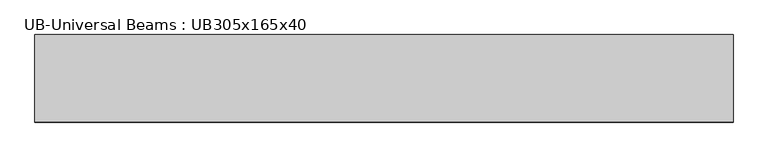
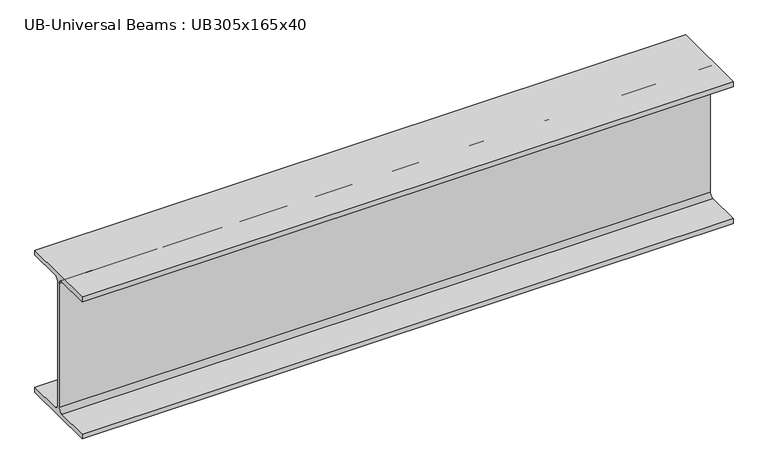
"""IFC4 building model written with IfcOpenShell, lengths in millimetres: beam geometry, UB-Universal Beams : UB305x165x40."""

from ifc_helpers import new_model, si_unit, point, frame, frame_2d, origin, place, context, project, spatial, polyline, circle_curve, trimmed, segment, composite_curve, outline, extrude, source, transform, mapped, element, save


def ub_universal_beams_ub305x165x40_9340f7ff(model_context):
    return source(origin(), model_context, "Body", "SweptSolid", [
        extrude(outline(composite_curve([segment(polyline([(82.5, -141.5), (82.5, -151.7), (-82.5, -151.7), (-82.5, -141.5), (-11.9, -141.5)]), True, "CONTINUOUS"), segment(trimmed(circle_curve(frame_2d((-11.9, -132.6)), 8.9), [point((-11.9, -141.5))], [point((-3.0, -132.6))], True, "CARTESIAN"), True, "CONTINUOUS"), segment(polyline([(-3.0, -132.6), (-3.0, 132.6)]), True, "CONTINUOUS"), segment(trimmed(circle_curve(frame_2d((-11.9, 132.6)), 8.9), [point((-3.0, 132.6))], [point((-11.9, 141.5))], True, "CARTESIAN"), True, "CONTINUOUS"), segment(polyline([(-11.9, 141.5), (-82.5, 141.5), (-82.5, 151.7), (82.5, 151.7), (82.5, 141.5), (11.9, 141.5)]), True, "CONTINUOUS"), segment(trimmed(circle_curve(frame_2d((11.9, 132.6)), 8.9), [point((11.9, 141.5))], [point((3.0, 132.6))], True, "CARTESIAN"), True, "CONTINUOUS"), segment(polyline([(3.0, 132.6), (3.0, -132.6)]), True, "CONTINUOUS"), segment(trimmed(circle_curve(frame_2d((11.9, -132.6)), 8.9), [point((3.0, -132.6))], [point((11.9, -141.5))], True, "CARTESIAN"), True, "CONTINUOUS"), segment(polyline([(11.9, -141.5), (82.5, -141.5)]), True, "CONTINUOUS")], self_intersect=False)), frame((-668.9, 0.0, 0.0), z_axis=(1.0, 0.0, 0.0), x_axis=(0.0, 1.0, 0.0)), (0.0, 0.0, 1.0), 1315.6),
    ])


if __name__ == "__main__":
    model = new_model("IFC4")
    model_context = context("Model", 3, world=origin())
    ifc_project = project(units=[si_unit("LENGTHUNIT", "METRE", prefix="MILLI")], contexts=[model_context])
    site = spatial("IfcSite", under=ifc_project)
    building = spatial("IfcBuilding", under=site)
    placement = place(None, origin())
    ub_universal_beams_ub305x165x40_shape = ub_universal_beams_ub305x165x40_9340f7ff(model_context)
    element("IfcBeam", 1, ObjectType="UB-Universal Beams : UB305x165x40", at=placement, inside=building, context=model_context, shape_type="MappedRepresentation", body=[
        mapped(ub_universal_beams_ub305x165x40_shape, transform((0.0, 0.0, 0.0), x_axis=(1.0, 0.0, 0.0), y_axis=(0.0, 1.0, 0.0), z_axis=(0.0, 0.0, 1.0))),
    ])
    save(model, "model.ifc")

# Revit data of these elements
# Type "UB-Universal Beams : UB305x165x40"
#   Section Name Key = "UB305X165X40"
#   Width = 16.5 cm
#   Web Thickness = 0.6 cm
#   Web Fillet = 0.89 cm
#   Warping Constant = 164000.0 cm⁶
#   Torsional Moment of Inertia = 14.70 cm⁴
#   Section Area = 51.3 cm²
#   Plastic Modulus weak axis = 142.0 cm³
#   Plastic Modulus strong axis = 623.0 cm³
#   Nominal Weight = 40.2999 kgf/m
#   Moment of Inertia weak axis = 764.00 cm⁴
#   Moment of Inertia strong axis = 8503.00 cm⁴
#   Height = 30.34 cm
#   Flange Thickness = 1.02 cm
#   Elastic Modulus weak axis = 92.6 cm³
#   Elastic Modulus strong axis = 560.0 cm³
#   Centroid Vertical = 15.17 cm
#   Centroid Horizontal = 8.25 cm
#   Bolt Spacing = 9.0 cm
#   Length [instance default] = 1500 mm
#   Structural Material [instance default] = Metal - Steel 43-275
#   Type Comments = ""
#   Assembly Code = ""
# Element 1 (IfcBeam, "UB-Universal Beams : UB305x165x40")
#   Materials on its faces: "Metal - Steel 43-275"
# Materials
#   "Metal - Steel 43-275": class "Metal", colour RGB 247 247 247, transparency 0, Cost = 0
